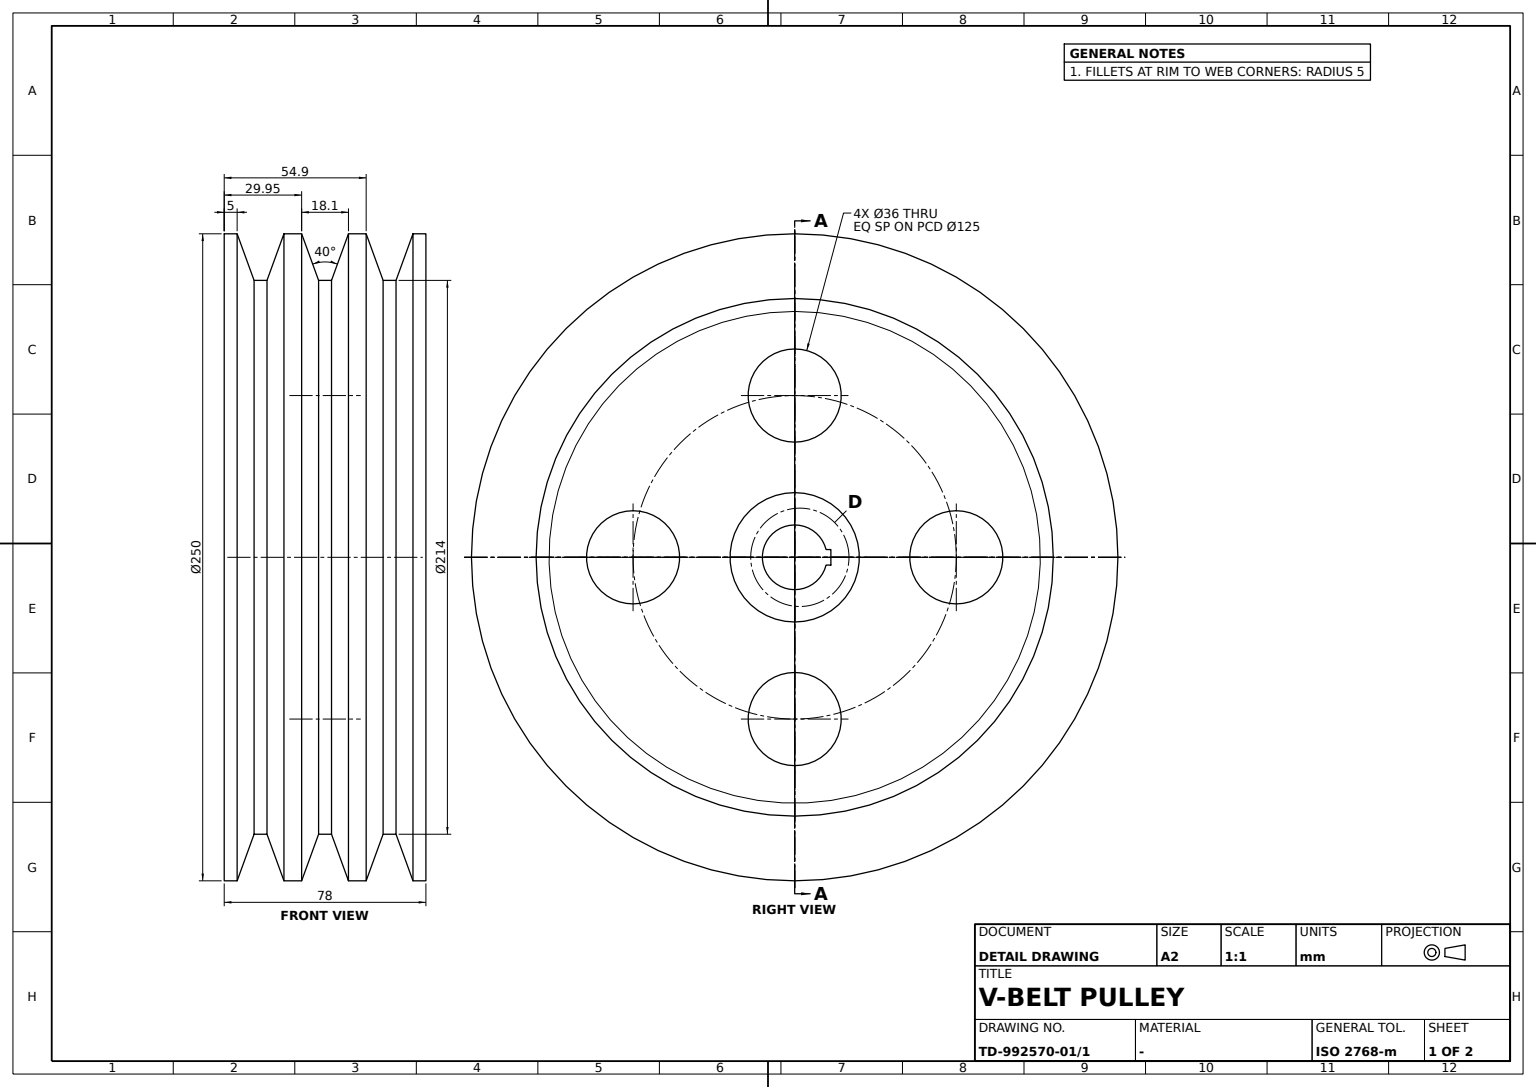
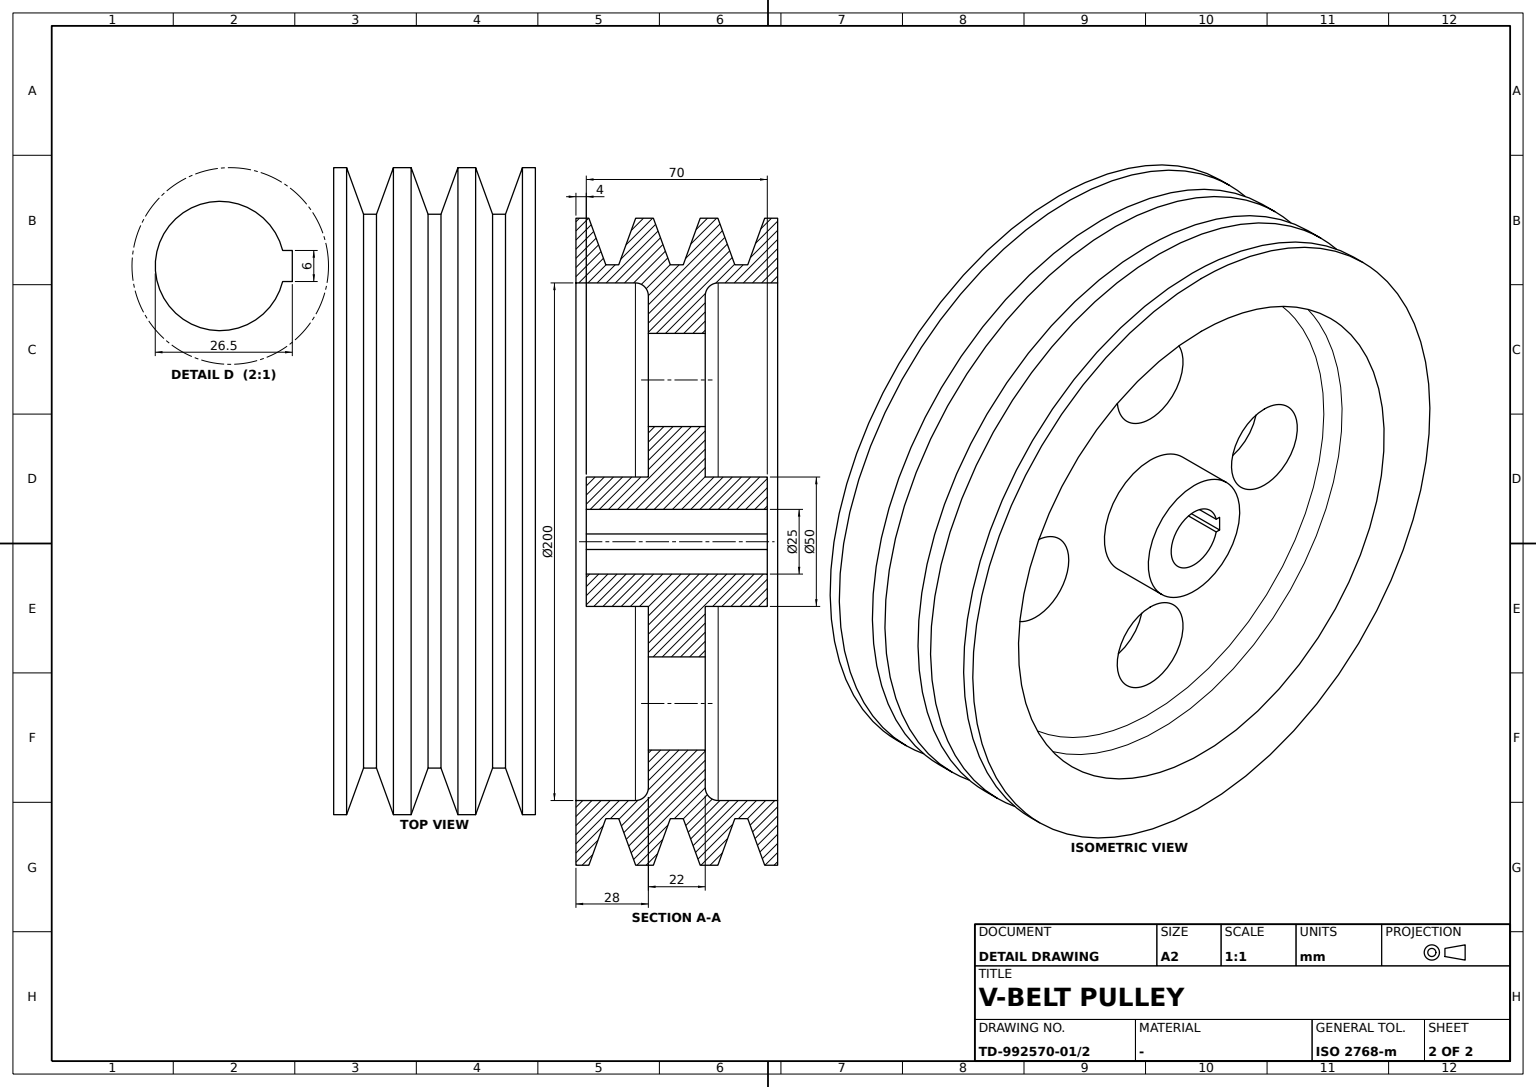
CATIA V5 part; units mm, degrees
sketch "Sketch1" plane through (0, 0, 0) normal (1, 0, 0) x (0, 1, 0)
  point P0 (-39, 125)
  line L0 (39, 125) -> (39, 100)
  line L1 (-39, 100) -> (-39, 125)
  point P1 (39, 125)
  point P2 (39, 0)
  point P3 (-39, 125)
  line L2 (-39, 125) -> (-34, 125)
  point P4 (-34, 125)
  line L3 (-34, 125) -> (-27.4485, 107)
  point P5 (-27.4485, 107)
  line L4 (-27.4485, 107) -> (-22.4485, 107)
  point P6 (-22.4485, 107)
  line L5 (-22.4485, 107) -> (-15.8971, 125)
  point P7 (-15.8971, 125)
  line L6 (0, -17.2623) -> (0, 173.9018) construction
  point P8 (0, -17.2623)
  line L7 (-15.8971, 125) -> (-9.0515, 125)
  point P9 (-9.0515, 125)
  line L8 (-9.0515, 125) -> (-2.5, 107)
  point P10 (-2.5, 107)
  line L9 (-2.5, 107) -> (0, 107)
  point P11 (0, 107)
  point P12 (34, 125)
  point P13 (39, 125)
  line L10 (39, 125) -> (34, 125)
  point P14 (27.4485, 107)
  line L11 (34, 125) -> (27.4485, 107)
  point P15 (22.4485, 107)
  line L12 (27.4485, 107) -> (22.4485, 107)
  point P16 (15.8971, 125)
  line L13 (22.4485, 107) -> (15.8971, 125)
  point P17 (9.0515, 125)
  line L14 (15.8971, 125) -> (9.0515, 125)
  point P18 (2.5, 107)
  line L15 (9.0515, 125) -> (2.5, 107)
  point P19 (0, 107)
  line L16 (2.5, 107) -> (0, 107)
  point P20 (24.9485, 107)
  line L17 (-24.9485, 107) -> (-24.9485, 137.999) construction
  point P21 (-24.9485, 107)
  line L18 (-39, 100) -> (-11, 100)
  point P22 (-11, 100)
  line L19 (-11, 100) -> (-11, 25)
  point P23 (-11, 25)
  line L20 (-11, 25) -> (-35, 25)
  point P24 (-35, 25)
  line L21 (-35, 25) -> (-35, 12.5)
  point P25 (-35, 12.5)
  line L22 (-35, 12.5) -> (0, 12.5)
  point P26 (0, 12.5)
  point P27 (-39, 100)
  point P28 (0, 12.5)
  point P29 (35, 12.5)
  line L23 (35, 12.5) -> (0, 12.5)
  point P30 (35, 25)
  line L24 (35, 25) -> (35, 12.5)
  point P31 (11, 25)
  line L25 (11, 25) -> (35, 25)
  point P32 (11, 100)
  line L26 (11, 100) -> (11, 25)
  point P33 (39, 100)
  line L27 (39, 100) -> (11, 100)
  dimension "angle L15 L8" = 40
  dimension "distance L4 L2" = 18
  dimension "length L10" = 5
  dimension "distance P10 P18" = 5
  dimension "length L4" = 5
  dimension "angle L3 L5" = 40
  dimension "distance L18 L2" = 25
  dimension "distance P1 P2" = 125
  dimension "distance L19 L26" = 22
  dimension "distance L21 L24" = 70
  dimension "distance L1 L0" = 78
  dimension "distance x axis L18" = 100
  dimension "distance x axis L23" = 12.5
  dimension "distance x axis L25" = 25
  constraint vertical L0 y-axis
  constraint vertical L1 y-axis
  constraint vertical L6 y-axis
  constraint vertical L17 y-axis
  constraint vertical L19 y-axis
  constraint vertical L21 y-axis
  constraint coincidence P2 x-axis
  constraint coincidence P7 L2
  constraint coincidence P8 y-axis
  constraint coincidence P10 L4
  constraint coincidence P11 L6
  constraint coincidence P3 P0
  constraint coincidence P13 P1
  constraint coincidence P26 L6
  constraint coincidence P11 P19
  constraint coincidence P26 P28
  constraint symmetry L1 L0 y-axis
  constraint symmetry P4 P12 L6
  constraint symmetry P3 P13 L6
  constraint symmetry L2 L10 L6
  constraint symmetry P5 P14 L6
  constraint symmetry L3 L11 L6
  constraint symmetry P6 P15 L6
  constraint symmetry L4 L12 L6
  constraint symmetry P7 P16 L6
  constraint symmetry L5 L13 L6
  constraint symmetry P9 P17 L6
  constraint symmetry L7 L14 L6
  constraint symmetry P10 P18 L6
  constraint symmetry L8 L15 L6
  constraint symmetry P11 P19 L6
  constraint symmetry L9 L16 L6
  constraint symmetry L3 L5 L17
  constraint symmetry P26 P28 L6
  constraint symmetry P25 P29 L6
  constraint symmetry L22 L23 L6
  constraint symmetry P24 P30 L6
  constraint symmetry L21 L24 L6
  constraint symmetry P23 P31 L6
  constraint symmetry L20 L25 L6
  constraint symmetry P22 P32 L6
  constraint symmetry L19 L26 L6
  constraint symmetry P27 P33 L6
  constraint symmetry L18 L27 L6
  constraint horizontal L2 x-axis
  constraint horizontal L4 x-axis
  constraint horizontal L7 x-axis
  constraint horizontal L9 x-axis
  constraint horizontal L18 x-axis
  constraint horizontal L20 x-axis
  constraint horizontal L22 x-axis
  constraint midpoint P20 L12
  constraint midpoint P21 L4
revolve "Shaft1" add sketch "Sketch1" angle 360 about axis through (0, 0, 0) along (0, 1, 0)
sketch "Sketch2" plane through (0, 11, 0) normal (0, 1, 0) x (-1, 0, 0)
  circle A0 centre (0, 0) radius 62.5 construction
  circle A1 centre (0, 62.5) radius 18
  point P0 (0, 62.5)
  circle A2 centre (-62.5, 0) radius 18
  circle A3 centre (0, -62.5) radius 18
  point P1 (62.5, 0)
  circle A4 centre (62.5, 0) radius 18
  dimension "radius A0" = 62.5
  dimension "radius A1" = 18
  dimension "distance P1 A4" = 18
  constraint coincidence P0 A0
  constraint coincidence P0 y-axis
extrude "Pocket1" cut sketch "Sketch2" against normal blind 24
sketch "Sketch3" plane through (0, 35, 0) normal (0, 1, 0) x (-1, 0, 0)
  point P0 (12.5, 0)
  line L0 (14, 3) -> (14, -3)
  line L1 (14, -3) -> (12.1347, -3)
  line L2 (12.1347, 3) -> (14, 3)
  point P1 (14, 3)
  point P2 (11, 3)
  circle A0 centre (0, 0) radius 12.5 construction
  arc A1 (12.1347, -3) -> (12.1347, 3) centre (0, 0) ccw
  point P3 (12.1347, 3)
  point P4 (12.1347, -3)
  dimension "length L0" = 6
  dimension "distance P2 P1" = 3
  constraint coincidence P0 x-axis
  constraint coincidence P0 A0
  constraint coincidence A0 P3
  constraint coincidence A0 P4
  constraint vertical L0 y-axis
  constraint horizontal L1 x-axis
  constraint horizontal L2 x-axis
  constraint equidistance L1 L2 P0
extrude "Pocket2" cut sketch "Sketch3" against normal blind 77
fillet "Fillet1" radius 5 1 edges at (0, 11, -100)
fillet "Fillet2" radius 5 1 edges at (0, -11, -100)
